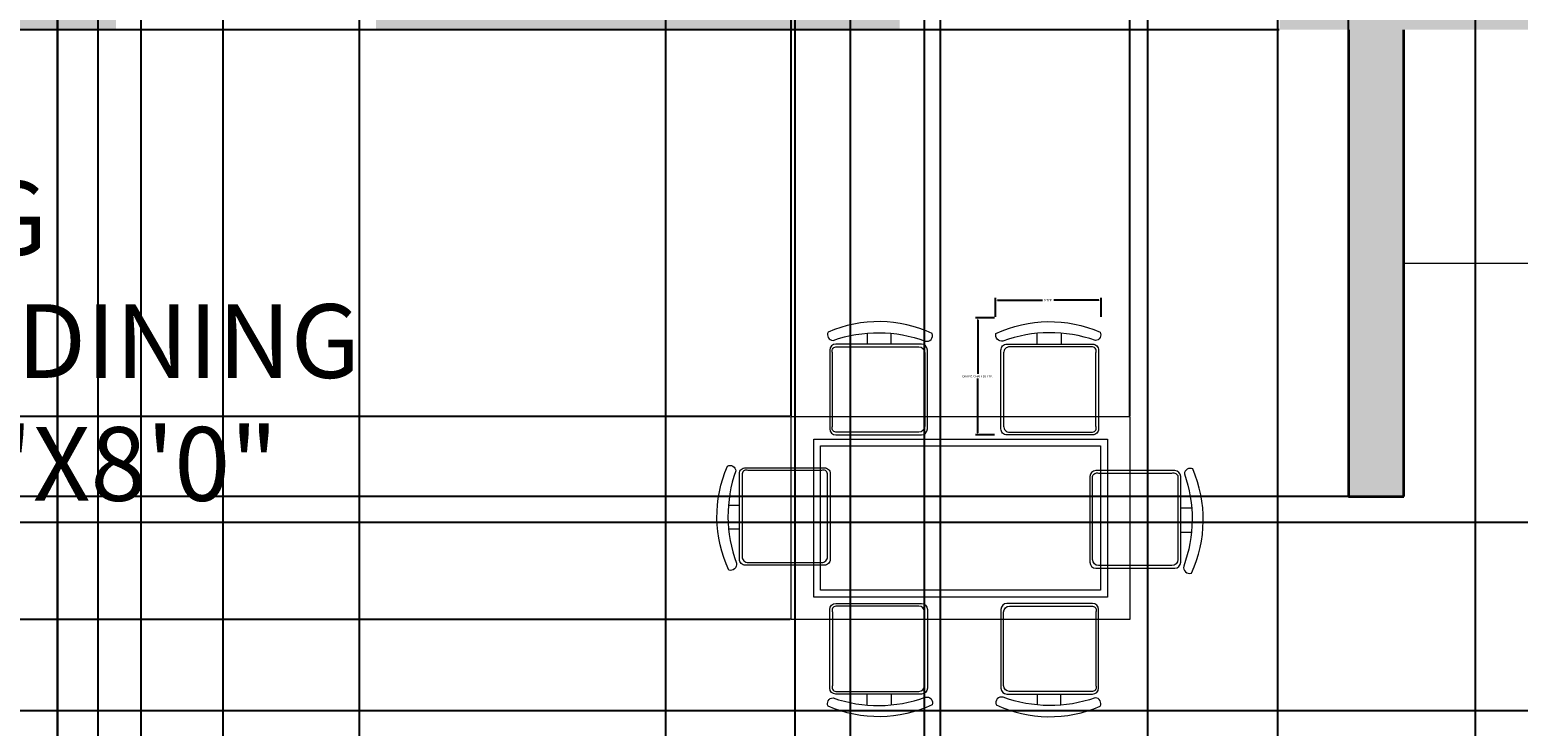
# Model space of a CAD drawing. Units: inches. Extents: x 2606 to 3027, y 1906 to 2463.
# Tile 6 of 10: x 2785 to 2906, y 2196 to 2253. Entities that reach past the tile are written whole.
import ezdxf

# ---------------------------------------------------------------- set-up
doc = ezdxf.new("R2010")
doc.units = ezdxf.units.IN
for name, color, linetype, lineweight in [('A-ANNO-DIMS', 2, 'Continuous', 18), ('A-AREA-IDEN', 7, 'Continuous', 18), ('A-FLOR-CASE', 8, 'Continuous', 18), ('A-FURN', 8, 'Continuous', 13), ('A-WALL', 7, 'Continuous', 35)]:
    doc.layers.add(name, color=color, linetype=linetype, lineweight=lineweight)
doc.layers.add('A-WALL-PATT', color=251, linetype='Continuous', lineweight=13, true_color=0x636466)
doc.styles.get("Standard").update_dxf_attribs({"font": 'arial.ttf'})
doc.dimstyles.get("Standard").update_dxf_attribs({"dimtxt": 0.18, "dimasz": 0.18, "dimexe": 0.18, "dimexo": 0.0625, "dimgap": 0.09, "dimtad": 0, "dimtih": 1, "dimtoh": 1, "dimdec": 4, "dimzin": 0, "dimdsep": 46, "dimtxsty": 'Standard', "dimcen": 0.09, "dimadec": 0, "dimazin": 0, "dimtfac": 1, "dimtdec": 4, "dimtofl": 0, "dimtmove": 0, "dimatfit": 3, "dimfxl": 1, "dimtolj": 1, "dimtzin": 0, "dimarcsym": 0})

# ---------------------------------------------------------------- blocks, each defined once
blk = doc.blocks.new('CHAIR-DINING')
for points in [[(0.59, 7.63, -0.578392), (0.02, 8.25, -0.214524), (8.49, 8.36, -0.552014), (8.1, 7.68, 0.175809), (0.59, 7.63)], [(7.88, 7.38, -0.414214), (8.36, 6.89), (8.36, 0.49, -0.414214), (7.88, 0), (0.91, 0, -0.414214), (0.42, 0.49), (0.42, 6.89, -0.414214), (0.91, 7.38), (7.88, 7.38)], [(3.36, 7.38), (3.36, 8.26, 0.064759)]]:
    blk.add_lwpolyline(points, format="xyb")
blk.add_lwpolyline([(5.31, 8.28), (5.31, 7.38)])
blk.add_lwpolyline([(7.87, 7.16), (1.13, 7.16, 0.414214), (0.64, 6.67), (0.64, 0.71, 0.414214), (1.13, 0.22), (7.87, 0.22, 0.512069), (8.14, 0.71), (8.14, 6.67, 0.512069)], format="xyb", close=True)
blk = doc.blocks.new('*D23')
at = {"layer": 'A-ANNO-DIMS', "color": 0, "lineweight": -2, "transparency": 16777216}
for p, q in [((2863.77, 2229.68), (2862.22, 2229.68)), ((2862.4, 2229.5), (2862.4, 2225.1)), ((2862.4, 2220.32), (2862.4, 2224.73)), ((2863.77, 2220.14), (2862.22, 2220.14))]:
    blk.add_line(p, q, dxfattribs=at)
at = {"layer": 'A-ANNO-DIMS', "color": 0, "transparency": 16777216}
for points in [[(2862.37, 2229.5), (2862.43, 2229.5), (2862.4, 2229.68)], [(2862.37, 2220.32), (2862.43, 2220.32), (2862.4, 2220.14)]]:
    blk.add_solid(points, dxfattribs=at)
at = {"layer": 'Defpoints', "color": 0, "transparency": 16777216}
for p in [(2862.4, 2229.68), (2863.84, 2229.68), (2863.84, 2220.14)]:
    blk.add_point(p, dxfattribs=at)
at = {"layer": 'A-ANNO-DIMS', "color": 0, "transparency": 16777216, "insert": (2862.4, 2224.91), "char_height": 0.18, "attachment_point": 5}
blk.add_mtext('\\A1;DINING CHAIR 10 TYP.', dxfattribs=at)
blk = doc.blocks.new('*D24')
at = {"layer": 'A-ANNO-DIMS', "color": 0, "lineweight": -2, "transparency": 16777216}
for p, q in [((2863.84, 2229.75), (2863.84, 2231.29)), ((2864.02, 2231.11), (2867.68, 2231.11)), ((2872.25, 2231.11), (2868.59, 2231.11)), ((2872.43, 2229.75), (2872.43, 2231.29))]:
    blk.add_line(p, q, dxfattribs=at)
at = {"layer": 'A-ANNO-DIMS', "color": 0, "transparency": 16777216}
for points in [[(2864.02, 2231.14), (2864.02, 2231.08), (2863.84, 2231.11)], [(2872.25, 2231.14), (2872.25, 2231.08), (2872.43, 2231.11)]]:
    blk.add_solid(points, dxfattribs=at)
at = {"layer": 'Defpoints', "color": 0, "transparency": 16777216}
for p in [(2872.43, 2231.11), (2863.84, 2229.68), (2872.43, 2229.68)]:
    blk.add_point(p, dxfattribs=at)
at = {"layer": 'A-ANNO-DIMS', "color": 0, "transparency": 16777216, "insert": (2868.13, 2231.11), "char_height": 0.18, "attachment_point": 5}
blk.add_mtext('\\A1;9 TYP.', dxfattribs=at)
blk = doc.blocks.new('*D34')
at = {"layer": 'A-ANNO-DIMS', "color": 0, "lineweight": -2, "transparency": 16777216}
for p, q in [((2787.56, 2118.27), (2787.56, 2433.99)), ((2787.74, 2433.81), (2817.34, 2433.81)), ((2847.38, 2433.81), (2817.78, 2433.81)), ((2847.56, 2118.27), (2847.56, 2433.99))]:
    blk.add_line(p, q, dxfattribs=at)
at = {"layer": 'A-ANNO-DIMS', "color": 0, "transparency": 16777216}
for points in [[(2787.74, 2433.84), (2787.74, 2433.78), (2787.56, 2433.81)], [(2847.38, 2433.84), (2847.38, 2433.78), (2847.56, 2433.81)]]:
    blk.add_solid(points, dxfattribs=at)
at = {"layer": 'Defpoints', "color": 0, "transparency": 16777216}
for p in [(2847.56, 2433.81), (2787.56, 2118.21), (2847.56, 2118.21)]:
    blk.add_point(p, dxfattribs=at)
at = {"layer": 'A-ANNO-DIMS', "color": 0, "transparency": 16777216, "insert": (2817.56, 2433.81), "char_height": 0.18, "attachment_point": 5}
blk.add_mtext('\\A1;60', dxfattribs=at)
blk = doc.blocks.new('*D35')
at = {"layer": 'A-ANNO-DIMS', "color": 0, "lineweight": -2, "transparency": 16777216}
for p, q in [((2801.04, 1993.17), (2801.04, 2433.99)), ((2801.22, 2433.81), (2818.82, 2433.81)), ((2836.86, 2433.81), (2819.26, 2433.81)), ((2837.04, 1993.17), (2837.04, 2433.99))]:
    blk.add_line(p, q, dxfattribs=at)
at = {"layer": 'A-ANNO-DIMS', "color": 0, "transparency": 16777216}
for points in [[(2801.22, 2433.84), (2801.22, 2433.78), (2801.04, 2433.81)], [(2836.86, 2433.84), (2836.86, 2433.78), (2837.04, 2433.81)]]:
    blk.add_solid(points, dxfattribs=at)
at = {"layer": 'Defpoints', "color": 0, "transparency": 16777216}
for p in [(2837.04, 2433.81), (2801.04, 1993.11), (2837.04, 1993.11)]:
    blk.add_point(p, dxfattribs=at)
at = {"layer": 'A-ANNO-DIMS', "color": 0, "transparency": 16777216, "insert": (2819.04, 2433.81), "char_height": 0.18, "attachment_point": 5}
blk.add_mtext('\\A1;36', dxfattribs=at)
blk = doc.blocks.new('*D36')
at = {"layer": 'A-ANNO-DIMS', "color": 0, "lineweight": -2, "transparency": 16777216}
for p, q in [((2787.56, 1993.17), (2787.56, 2433.99)), ((2787.74, 2433.81), (2793.85, 2433.81)), ((2800.86, 2433.81), (2794.76, 2433.81)), ((2801.04, 1993.17), (2801.04, 2433.99))]:
    blk.add_line(p, q, dxfattribs=at)
at = {"layer": 'A-ANNO-DIMS', "color": 0, "transparency": 16777216}
for points in [[(2787.74, 2433.84), (2787.74, 2433.78), (2787.56, 2433.81)], [(2800.86, 2433.84), (2800.86, 2433.78), (2801.04, 2433.81)]]:
    blk.add_solid(points, dxfattribs=at)
at = {"layer": 'Defpoints', "color": 0, "transparency": 16777216}
for p in [(2787.56, 2433.81), (2787.56, 1993.11), (2801.04, 1993.11)]:
    blk.add_point(p, dxfattribs=at)
at = {"layer": 'A-ANNO-DIMS', "color": 0, "transparency": 16777216, "insert": (2794.3, 2433.81), "char_height": 0.18, "attachment_point": 5}
blk.add_mtext('\\A1;13.478', dxfattribs=at)
blk = doc.blocks.new('*D38')
at = {"layer": 'A-ANNO-DIMS', "color": 0, "lineweight": -2, "transparency": 16777216}
for p, q in [((2783.06, 1993.17), (2783.06, 2433.99)), ((2783.24, 2433.81), (2785.05, 2433.81)), ((2787.38, 2433.81), (2785.57, 2433.81)), ((2787.56, 1993.17), (2787.56, 2433.99))]:
    blk.add_line(p, q, dxfattribs=at)
at = {"layer": 'A-ANNO-DIMS', "color": 0, "transparency": 16777216}
for points in [[(2783.24, 2433.84), (2783.24, 2433.78), (2783.06, 2433.81)], [(2787.38, 2433.84), (2787.38, 2433.78), (2787.56, 2433.81)]]:
    blk.add_solid(points, dxfattribs=at)
at = {"layer": 'Defpoints', "color": 0, "transparency": 16777216}
for p in [(2787.56, 2433.81), (2783.06, 1993.11), (2787.56, 1993.11)]:
    blk.add_point(p, dxfattribs=at)
at = {"layer": 'A-ANNO-DIMS', "color": 0, "transparency": 16777216, "insert": (2785.31, 2433.81), "char_height": 0.18, "attachment_point": 5}
blk.add_mtext('\\A1;4.5', dxfattribs=at)
blk = doc.blocks.new('*D43')
at = {"layer": 'A-ANNO-DIMS', "color": 0, "lineweight": -2, "transparency": 16777216}
for p, q in [((2794.34, 2257.55), (2794.34, 1965.23)), ((2812.09, 2257.55), (2812.09, 1965.23)), ((2794.52, 1965.41), (2802.76, 1965.41)), ((2811.91, 1965.41), (2803.67, 1965.41))]:
    blk.add_line(p, q, dxfattribs=at)
at = {"layer": 'A-ANNO-DIMS', "color": 0, "transparency": 16777216}
for points in [[(2794.52, 1965.44), (2794.52, 1965.38), (2794.34, 1965.41)], [(2811.91, 1965.44), (2811.91, 1965.38), (2812.09, 1965.41)]]:
    blk.add_solid(points, dxfattribs=at)
at = {"layer": 'Defpoints', "color": 0, "transparency": 16777216}
for p in [(2794.34, 2257.61), (2812.09, 2257.61), (2812.09, 1965.41)]:
    blk.add_point(p, dxfattribs=at)
at = {"layer": 'A-ANNO-DIMS', "color": 0, "transparency": 16777216, "insert": (2803.22, 1965.41), "char_height": 0.18, "attachment_point": 5}
blk.add_mtext('\\A1;17.756', dxfattribs=at)
blk = doc.blocks.new('*D46')
at = {"layer": 'A-ANNO-DIMS', "color": 0, "lineweight": -2, "transparency": 16777216}
for p, q in [((2859.37, 2154.92), (2859.37, 2433.99)), ((2859.55, 2433.81), (2872.63, 2433.81)), ((2886.63, 2433.81), (2873.56, 2433.81)), ((2886.81, 2157.17), (2886.81, 2433.99))]:
    blk.add_line(p, q, dxfattribs=at)
at = {"layer": 'A-ANNO-DIMS', "color": 0, "transparency": 16777216}
for points in [[(2859.55, 2433.84), (2859.55, 2433.78), (2859.37, 2433.81)], [(2886.63, 2433.84), (2886.63, 2433.78), (2886.81, 2433.81)]]:
    blk.add_solid(points, dxfattribs=at)
at = {"layer": 'Defpoints', "color": 0, "transparency": 16777216}
for p in [(2886.81, 2433.81), (2886.81, 2157.11), (2859.37, 2154.86)]:
    blk.add_point(p, dxfattribs=at)
at = {"layer": 'A-ANNO-DIMS', "color": 0, "transparency": 16777216, "insert": (2873.09, 2433.81), "char_height": 0.18, "attachment_point": 5}
blk.add_mtext('\\A1;27.443', dxfattribs=at)
blk = doc.blocks.new('*D48')
at = {"layer": 'A-ANNO-DIMS', "color": 0, "lineweight": -2, "transparency": 16777216}
for p, q in [((2858.07, 2028.17), (2858.07, 2433.99)), ((2858.25, 2433.81), (2866.77, 2433.81)), ((2876.06, 2433.81), (2867.54, 2433.81)), ((2876.24, 2028.17), (2876.24, 2433.99))]:
    blk.add_line(p, q, dxfattribs=at)
at = {"layer": 'A-ANNO-DIMS', "color": 0, "transparency": 16777216}
for points in [[(2858.25, 2433.84), (2858.25, 2433.78), (2858.07, 2433.81)], [(2876.06, 2433.84), (2876.06, 2433.78), (2876.24, 2433.81)]]:
    blk.add_solid(points, dxfattribs=at)
at = {"layer": 'Defpoints', "color": 0, "transparency": 16777216}
for p in [(2876.24, 2433.81), (2858.07, 2028.11), (2876.24, 2028.11)]:
    blk.add_point(p, dxfattribs=at)
at = {"layer": 'A-ANNO-DIMS', "color": 0, "transparency": 16777216, "insert": (2867.16, 2433.81), "char_height": 0.18, "attachment_point": 5}
blk.add_mtext('\\A1;18.17', dxfattribs=at)
blk = doc.blocks.new('*D52')
at = {"layer": 'A-ANNO-DIMS', "color": 0, "lineweight": -2, "transparency": 16777216}
for p, q in [((2787.56, 2257.55), (2787.56, 1965.23)), ((2794.34, 2257.55), (2794.34, 1965.23)), ((2787.74, 1965.41), (2790.56, 1965.41)), ((2794.16, 1965.41), (2791.34, 1965.41))]:
    blk.add_line(p, q, dxfattribs=at)
at = {"layer": 'A-ANNO-DIMS', "color": 0, "transparency": 16777216}
for points in [[(2787.74, 1965.44), (2787.74, 1965.38), (2787.56, 1965.41)], [(2794.16, 1965.44), (2794.16, 1965.38), (2794.34, 1965.41)]]:
    blk.add_solid(points, dxfattribs=at)
at = {"layer": 'Defpoints', "color": 0, "transparency": 16777216}
for p in [(2787.56, 2257.61), (2794.34, 2257.61), (2794.34, 1965.41)]:
    blk.add_point(p, dxfattribs=at)
at = {"layer": 'A-ANNO-DIMS', "color": 0, "transparency": 16777216, "insert": (2790.95, 1965.41), "char_height": 0.18, "attachment_point": 5}
blk.add_mtext('\\A1;6.776', dxfattribs=at)
blk = doc.blocks.new('*D55')
at = {"layer": 'A-ANNO-DIMS', "color": 0, "lineweight": -2, "transparency": 16777216}
for p, q in [((2852.06, 2152.67), (2852.06, 2433.99)), ((2852.24, 2433.81), (2855.32, 2433.81)), ((2859.19, 2433.81), (2856.11, 2433.81)), ((2859.37, 2154.92), (2859.37, 2433.99))]:
    blk.add_line(p, q, dxfattribs=at)
at = {"layer": 'A-ANNO-DIMS', "color": 0, "transparency": 16777216}
for points in [[(2852.24, 2433.84), (2852.24, 2433.78), (2852.06, 2433.81)], [(2859.19, 2433.84), (2859.19, 2433.78), (2859.37, 2433.81)]]:
    blk.add_solid(points, dxfattribs=at)
at = {"layer": 'Defpoints', "color": 0, "transparency": 16777216}
for p in [(2859.37, 2433.81), (2859.37, 2154.86), (2852.06, 2152.61)]:
    blk.add_point(p, dxfattribs=at)
at = {"layer": 'A-ANNO-DIMS', "color": 0, "transparency": 16777216, "insert": (2855.72, 2433.81), "char_height": 0.18, "attachment_point": 5}
blk.add_mtext('\\A1;7.306', dxfattribs=at)
blk = doc.blocks.new('*D57')
at = {"layer": 'A-ANNO-DIMS', "color": 0, "lineweight": -2, "transparency": 16777216}
for p, q in [((2876.24, 2028.17), (2876.24, 2433.99)), ((2876.42, 2433.81), (2889.17, 2433.81)), ((2902.71, 2433.81), (2889.96, 2433.81)), ((2902.89, 2028.17), (2902.89, 2433.99))]:
    blk.add_line(p, q, dxfattribs=at)
at = {"layer": 'A-ANNO-DIMS', "color": 0, "transparency": 16777216}
for points in [[(2876.42, 2433.84), (2876.42, 2433.78), (2876.24, 2433.81)], [(2902.71, 2433.84), (2902.71, 2433.78), (2902.89, 2433.81)]]:
    blk.add_solid(points, dxfattribs=at)
at = {"layer": 'Defpoints', "color": 0, "transparency": 16777216}
for p in [(2902.89, 2433.81), (2876.24, 2028.11), (2902.89, 2028.11)]:
    blk.add_point(p, dxfattribs=at)
at = {"layer": 'A-ANNO-DIMS', "color": 0, "transparency": 16777216, "insert": (2889.57, 2433.81), "char_height": 0.18, "attachment_point": 5}
blk.add_mtext('\\A1;26.65', dxfattribs=at)
blk = doc.blocks.new('*D59')
at = {"layer": 'A-ANNO-DIMS', "color": 0, "lineweight": -2, "transparency": 16777216}
for p, q in [((2726.47, 2213.03), (3000.44, 2213.03)), ((3000.26, 2212.85), (3000.26, 2205.56)), ((3000.26, 2197.9), (3000.26, 2205.2)), ((2726.47, 2197.72), (3000.44, 2197.72))]:
    blk.add_line(p, q, dxfattribs=at)
at = {"layer": 'A-ANNO-DIMS', "color": 0, "transparency": 16777216}
for points in [[(3000.23, 2212.85), (3000.29, 2212.85), (3000.26, 2213.03)], [(3000.23, 2197.9), (3000.29, 2197.9), (3000.26, 2197.72)]]:
    blk.add_solid(points, dxfattribs=at)
at = {"layer": 'Defpoints', "color": 0, "transparency": 16777216}
for p in [(2726.4, 2213.03), (3000.26, 2213.03), (2726.4, 2197.72)]:
    blk.add_point(p, dxfattribs=at)
at = {"layer": 'A-ANNO-DIMS', "color": 0, "transparency": 16777216, "insert": (3000.26, 2205.38), "char_height": 0.18, "attachment_point": 5}
blk.add_mtext('\\A1;15.31', dxfattribs=at)
blk = doc.blocks.new('*D61')
at = {"layer": 'A-ANNO-DIMS', "color": 0, "lineweight": -2, "transparency": 16777216}
for p, q in [((2696.29, 2197.72), (3000.44, 2197.72)), ((3000.26, 2197.54), (3000.26, 2190.63)), ((3000.26, 2183.36), (3000.26, 2190.27)), ((2696.84, 2183.18), (3000.44, 2183.18))]:
    blk.add_line(p, q, dxfattribs=at)
at = {"layer": 'A-ANNO-DIMS', "color": 0, "transparency": 16777216}
for points in [[(3000.23, 2197.54), (3000.29, 2197.54), (3000.26, 2197.72)], [(3000.23, 2183.36), (3000.29, 2183.36), (3000.26, 2183.18)]]:
    blk.add_solid(points, dxfattribs=at)
at = {"layer": 'Defpoints', "color": 0, "transparency": 16777216}
for p in [(2696.23, 2197.72), (3000.26, 2197.72), (2696.78, 2183.18)]:
    blk.add_point(p, dxfattribs=at)
at = {"layer": 'A-ANNO-DIMS', "color": 0, "transparency": 16777216, "insert": (3000.26, 2190.45), "char_height": 0.18, "attachment_point": 5}
blk.add_mtext('\\A1;14.545', dxfattribs=at)
blk = doc.blocks.new('*D68')
at = {"layer": 'A-ANNO-DIMS', "color": 0, "lineweight": -2, "transparency": 16777216}
for p, q in [((2897, 2215.13), (2634.68, 2215.13)), ((2634.86, 2214.95), (2634.86, 2194.85)), ((2634.86, 2174.38), (2634.86, 2194.48)), ((2897, 2174.2), (2634.68, 2174.2))]:
    blk.add_line(p, q, dxfattribs=at)
at = {"layer": 'A-ANNO-DIMS', "color": 0, "transparency": 16777216}
for points in [[(2634.83, 2214.95), (2634.89, 2214.95), (2634.86, 2215.13)], [(2634.83, 2174.38), (2634.89, 2174.38), (2634.86, 2174.2)]]:
    blk.add_solid(points, dxfattribs=at)
at = {"layer": 'Defpoints', "color": 0, "transparency": 16777216}
for p in [(2897.06, 2215.13), (2634.86, 2174.2), (2897.06, 2174.2)]:
    blk.add_point(p, dxfattribs=at)
at = {"layer": 'A-ANNO-DIMS', "color": 0, "transparency": 16777216, "insert": (2634.86, 2194.66), "char_height": 0.18, "attachment_point": 5}
blk.add_mtext('\\A1;40.94', dxfattribs=at)
blk = doc.blocks.new('*D70')
at = {"layer": 'A-ANNO-DIMS', "color": 0, "lineweight": -2, "transparency": 16777216}
for p, q in [((2847.23, 2221.7), (2847.23, 2433.99)), ((2847.41, 2433.81), (2860.54, 2433.81)), ((2874.6, 2433.81), (2861.47, 2433.81)), ((2874.78, 2221.7), (2874.78, 2433.99))]:
    blk.add_line(p, q, dxfattribs=at)
at = {"layer": 'A-ANNO-DIMS', "color": 0, "transparency": 16777216}
for points in [[(2847.41, 2433.84), (2847.41, 2433.78), (2847.23, 2433.81)], [(2874.6, 2433.84), (2874.6, 2433.78), (2874.78, 2433.81)]]:
    blk.add_solid(points, dxfattribs=at)
at = {"layer": 'Defpoints', "color": 0, "transparency": 16777216}
for p in [(2874.78, 2433.81), (2847.23, 2221.64), (2874.78, 2221.64)]:
    blk.add_point(p, dxfattribs=at)
at = {"layer": 'A-ANNO-DIMS', "color": 0, "transparency": 16777216, "insert": (2861, 2433.81), "char_height": 0.18, "attachment_point": 5}
blk.add_mtext('\\A1;27.555', dxfattribs=at)
blk = doc.blocks.new('*D71')
at = {"layer": 'A-ANNO-DIMS', "color": 0, "lineweight": -2, "transparency": 16777216}
for p, q in [((2847.16, 2221.64), (2634.68, 2221.64)), ((2634.86, 2221.46), (2634.86, 2213.56)), ((2634.86, 2205.29), (2634.86, 2213.19)), ((2847.16, 2205.11), (2634.68, 2205.11))]:
    blk.add_line(p, q, dxfattribs=at)
at = {"layer": 'A-ANNO-DIMS', "color": 0, "transparency": 16777216}
for points in [[(2634.83, 2221.46), (2634.89, 2221.46), (2634.86, 2221.64)], [(2634.83, 2205.29), (2634.89, 2205.29), (2634.86, 2205.11)]]:
    blk.add_solid(points, dxfattribs=at)
at = {"layer": 'Defpoints', "color": 0, "transparency": 16777216}
for p in [(2847.23, 2221.64), (2634.86, 2205.11), (2847.23, 2205.11)]:
    blk.add_point(p, dxfattribs=at)
at = {"layer": 'A-ANNO-DIMS', "color": 0, "transparency": 16777216, "insert": (2634.86, 2213.37), "char_height": 0.18, "attachment_point": 5}
blk.add_mtext('\\A1;16.533', dxfattribs=at)
blk = doc.blocks.new('*D72')
at = {"layer": 'A-ANNO-DIMS', "color": 0, "lineweight": -2, "transparency": 16777216}
for p, q in [((2874.78, 2221.7), (2874.78, 2433.99)), ((2874.96, 2433.81), (2883.22, 2433.81)), ((2892.38, 2433.81), (2884.13, 2433.81)), ((2892.56, 2215.2), (2892.56, 2433.99))]:
    blk.add_line(p, q, dxfattribs=at)
at = {"layer": 'A-ANNO-DIMS', "color": 0, "transparency": 16777216}
for points in [[(2874.96, 2433.84), (2874.96, 2433.78), (2874.78, 2433.81)], [(2892.38, 2433.84), (2892.38, 2433.78), (2892.56, 2433.81)]]:
    blk.add_solid(points, dxfattribs=at)
at = {"layer": 'Defpoints', "color": 0, "transparency": 16777216}
for p in [(2892.56, 2433.81), (2874.78, 2221.64), (2892.56, 2215.13)]:
    blk.add_point(p, dxfattribs=at)
at = {"layer": 'A-ANNO-DIMS', "color": 0, "transparency": 16777216, "insert": (2883.67, 2433.81), "char_height": 0.18, "attachment_point": 5}
blk.add_mtext('\\A1;17.783', dxfattribs=at)
blk = doc.blocks.new('*D73')
at = {"layer": 'A-ANNO-DIMS', "color": 0, "lineweight": -2, "transparency": 16777216}
for p, q in [((2886.91, 2253.11), (2634.68, 2253.11)), ((2634.86, 2252.93), (2634.86, 2237.56)), ((2634.86, 2221.82), (2634.86, 2237.19)), ((2847.16, 2221.64), (2634.68, 2221.64))]:
    blk.add_line(p, q, dxfattribs=at)
at = {"layer": 'A-ANNO-DIMS', "color": 0, "transparency": 16777216}
for points in [[(2634.83, 2252.93), (2634.89, 2252.93), (2634.86, 2253.11)], [(2634.83, 2221.82), (2634.89, 2221.82), (2634.86, 2221.64)]]:
    blk.add_solid(points, dxfattribs=at)
at = {"layer": 'Defpoints', "color": 0, "transparency": 16777216}
for p in [(2634.86, 2253.11), (2886.97, 2253.11), (2847.23, 2221.64)]:
    blk.add_point(p, dxfattribs=at)
at = {"layer": 'A-ANNO-DIMS', "color": 0, "transparency": 16777216, "insert": (2634.86, 2237.37), "char_height": 0.18, "attachment_point": 5}
blk.add_mtext('\\A1;31.47', dxfattribs=at)
blk = doc.blocks.new('*D83')
at = {"layer": 'A-ANNO-DIMS', "color": 0, "lineweight": -2, "transparency": 16777216}
for p, q in [((2787.56, 2327.05), (2787.56, 1965.23)), ((2790.85, 2327.05), (2790.85, 1965.23)), ((2787.74, 1965.41), (2788.88, 1965.41)), ((2790.67, 1965.41), (2789.53, 1965.41))]:
    blk.add_line(p, q, dxfattribs=at)
at = {"layer": 'A-ANNO-DIMS', "color": 0, "transparency": 16777216}
for points in [[(2787.74, 1965.44), (2787.74, 1965.38), (2787.56, 1965.41)], [(2790.67, 1965.44), (2790.67, 1965.38), (2790.85, 1965.41)]]:
    blk.add_solid(points, dxfattribs=at)
at = {"layer": 'Defpoints', "color": 0, "transparency": 16777216}
for p in [(2787.56, 2327.11), (2790.85, 2327.11), (2790.85, 1965.41)]:
    blk.add_point(p, dxfattribs=at)
at = {"layer": 'A-ANNO-DIMS', "color": 0, "transparency": 16777216, "insert": (2789.21, 1965.41), "char_height": 0.18, "attachment_point": 5}
blk.add_mtext('\\A1;3.29', dxfattribs=at)

msp = doc.modelspace()

# ---------------------------------------------------------------- hatches: boundary and pattern name
at = {"layer": 'A-WALL-PATT'}
h = msp.add_hatch(color=256, dxfattribs=at)
h.dxf.hatch_style = 1
h.paths.add_polyline_path([(2667.063, 2401.6097), (2691.9697, 2401.6097), (2691.9697, 2406.1097), (2691.9697, 2410.6097), (2658.063, 2410.6097), (2658.063, 2238.7051), (2667.063, 2238.7051)])
h.paths.add_polyline_path([(2804.9965, 2406.1097), (2804.9965, 2410.6097), (2751.9697, 2410.6097), (2751.9697, 2401.6097), (2783.063, 2401.6097), (2783.063, 2257.6097), (2778.6739, 2257.6097), (2778.6739, 2253.1097), (2792.3386, 2253.1097), (2792.3386, 2255.3597), (2792.3386, 2257.6097), (2787.563, 2257.6097), (2787.563, 2327.1097), (2847.563, 2327.1097), (2847.563, 2331.6097), (2787.563, 2331.6097), (2787.563, 2401.6097), (2804.9965, 2401.6097)])
h.paths.add_polyline_path([(2889.6183, 2406.1097), (2889.6183, 2410.6097), (2828.9965, 2410.6097), (2828.9965, 2401.6097), (2831.8174, 2401.6097), (2847.563, 2401.6097), (2847.563, 2357.8311), (2849.813, 2357.8311), (2852.063, 2357.8311), (2852.063, 2401.6097), (2889.6183, 2401.6097)])
h.paths.add_polyline_path([(2977.063, 2410.6097), (2949.6183, 2410.6097), (2949.6183, 2401.6097), (2968.063, 2401.6097), (2968.063, 2157.1097), (2897.063, 2157.1097), (2897.063, 2174.1966), (2892.563, 2174.1966), (2892.563, 2157.1097), (2886.8122, 2157.1097), (2886.8122, 2152.6097), (2968.063, 2152.6097), (2968.063, 2032.6097), (2950.8911, 2032.6097), (2950.8911, 2028.1097), (2968.063, 2028.1097), (2968.063, 1993.1097), (2852.063, 1993.1097), (2852.063, 2028.1097), (2856.0743, 2028.1097), (2856.0743, 2030.3597), (2856.0743, 2032.6097), (2852.063, 2032.6097), (2852.063, 2152.6097), (2857.369, 2152.6097), (2857.369, 2154.8597), (2857.369, 2157.1097), (2847.563, 2157.1097), (2847.563, 2152.6097), (2847.563, 1993.1097), (2837.0415, 1993.1097), (2837.0415, 1988.6097), (2977.063, 1988.6097)])
h.paths.add_polyline_path([(2968.063, 2257.6097), (2886.9679, 2257.6097), (2886.9679, 2253.1097), (2892.563, 2253.1097), (2892.563, 2215.1332), (2897.063, 2215.1332), (2897.063, 2253.1097), (2968.063, 2253.1097)], flags=17)
h.paths.add_polyline_path([(2856.057, 2255.3597), (2856.057, 2257.6097), (2852.063, 2257.6097), (2852.063, 2336.7476), (2849.813, 2336.7476), (2847.563, 2336.7476), (2847.563, 2331.6097), (2847.563, 2327.1097), (2847.563, 2257.6097), (2813.482, 2257.6097), (2813.482, 2253.1097), (2856.057, 2253.1097)])
h.paths.add_polyline_path([(2748.8874, 2255.3597), (2748.8874, 2257.6097), (2667.063, 2257.6097), (2667.063, 2253.1097), (2748.8874, 2253.1097)])
h.paths.add_polyline_path([(2667.063, 2152.6097), (2744.8238, 2152.6097), (2744.8238, 2154.8597), (2744.8238, 2157.1097), (2667.063, 2157.1097), (2667.063, 2178.7051), (2658.063, 2178.7051), (2658.063, 1988.6097), (2801.0415, 1988.6097), (2801.0415, 1990.8597), (2801.0415, 1993.1097), (2787.563, 1993.1097), (2787.563, 2157.1097), (2777.1295, 2157.1097), (2777.1295, 2152.6097), (2783.063, 2152.6097), (2783.063, 2032.6097), (2778.4484, 2032.6097), (2778.4484, 2028.1097), (2783.063, 2028.1097), (2783.063, 1993.1097), (2667.063, 1993.1097), (2667.063, 2028.1097), (2680.1652, 2028.1097), (2680.1652, 2030.3597), (2680.1652, 2032.6097), (2667.063, 2032.6097)])
h.paths.add_polyline_path([(2755.4074, 2032.6097), (2728.1652, 2032.6097), (2728.1652, 2028.1097), (2755.4074, 2028.1097), (2755.4074, 2030.3597)], flags=17)
h.paths.add_polyline_path([(2902.8911, 2030.3597), (2902.8911, 2032.6097), (2877.6885, 2032.6097), (2877.6885, 2028.1097), (2902.8911, 2028.1097)], flags=17)
h.paths.add_polyline_path([(2810.2211, 2267.221), (2851.2716, 2267.221), (2851.2716, 2289.6098), (2810.2211, 2289.6098)], flags=9)

# ---------------------------------------------------------------- linework, layer by layer
at = {"layer": 'A-FLOR-CASE'}
msp.add_line((2897.063, 2234.1214), (2944.3333, 2234.1214), dxfattribs=at)
at = {"layer": 'A-FURN'}
for points in [[(2850.6334, 2227.8254, -0.17580919), (2858.1386, 2227.7686, 0.57839206), (2858.7071, 2228.3938, 0.21452438), (2850.2354, 2228.5075, 0.55201397), (2850.6334, 2227.8254, -0.06507904)], [(2855.3728, 2227.5242), (2855.3728, 2228.4054, -0.06475861)], [(2857.8202, 2227.5242), (2850.8526, 2227.5242, 0.41421356), (2850.3651, 2227.0368), (2850.3651, 2220.6302, 0.41421356), (2850.8526, 2220.1427), (2857.8202, 2220.1427, 0.41421356), (2858.3076, 2220.6302), (2858.3076, 2227.0368, 0.41421356), (2857.8202, 2227.5242)], [(2878.9056, 2216.7489, 0.41421356), (2878.4182, 2217.2363), (2872.0116, 2217.2363, 0.41421356), (2871.5242, 2216.7489), (2871.5242, 2209.7813, 0.41421356), (2872.0116, 2209.2938), (2878.4182, 2209.2938, 0.41421356), (2878.9056, 2209.7813), (2878.9056, 2216.7489)], [(2879.2069, 2216.9681, -0.17580919), (2879.15, 2209.4629, 0.57839206), (2879.7752, 2208.8943, 0.21452438), (2879.8889, 2217.3661, 0.55201397), (2879.2069, 2216.9681, -0.06507904)], [(2878.9056, 2212.2286), (2879.7868, 2212.2286, -0.06475861)], [(2857.8202, 2199.0455), (2850.8526, 2199.0455, -0.41421356), (2850.3651, 2199.533), (2850.3651, 2205.9395, -0.41421356), (2850.8526, 2206.427), (2857.8202, 2206.427, -0.41421356), (2858.3076, 2205.9395), (2858.3076, 2199.533, -0.41421356), (2857.8202, 2199.0455)], [(2871.743, 2199.0455, 0.41421356), (2872.2304, 2199.533), (2872.2304, 2205.9395, 0.41421356), (2871.743, 2206.427), (2864.7754, 2206.427, 0.41421356), (2864.2879, 2205.9395), (2864.2879, 2199.533, 0.41421356), (2864.7754, 2199.0455), (2871.743, 2199.0455)], [(2858.1386, 2198.8011, -0.57839206), (2858.7071, 2198.1759, -0.21452438), (2850.2354, 2198.0622, -0.55201397), (2850.6334, 2198.7443, 0.17580929), (2858.1386, 2198.8011)], [(2855.3728, 2199.0455), (2855.3728, 2198.1643, 0.06475861)], [(2871.9622, 2198.7443, -0.17580928), (2864.457, 2198.8011, 0.57839206), (2863.8884, 2198.1759, 0.21452438), (2872.3602, 2198.0622, 0.55201397), (2871.9622, 2198.7443, -0.06507904)], [(2867.2228, 2199.0455), (2867.2228, 2198.1643, -0.06475861)]]:
    msp.add_lwpolyline(points, format="xyb", dxfattribs=at)
for points in [[(2853.4225, 2228.4214), (2853.4225, 2227.5242)], [(2879.8028, 2214.179), (2878.9056, 2214.179)], [(2853.4225, 2198.1483), (2853.4225, 2199.0455)], [(2869.1731, 2198.1483), (2869.1731, 2199.0455)]]:
    msp.add_lwpolyline(points, dxfattribs=at)
for points in [[(2850.8555, 2227.3046), (2857.6005, 2227.3046, -0.41421356), (2858.088, 2226.8171), (2858.088, 2220.8498, -0.41421356), (2857.6005, 2220.3623), (2850.8555, 2220.3623, -0.51206948), (2850.5847, 2220.8498), (2850.5847, 2226.8171, -0.51206948)], [(2878.686, 2216.7459), (2878.686, 2210.0009, -0.41421356), (2878.1986, 2209.5134), (2872.2312, 2209.5134, -0.41421356), (2871.7438, 2210.0009), (2871.7438, 2216.7459, -0.51206948), (2872.2312, 2217.0167), (2878.1986, 2217.0167, -0.51206948)], [(2850.8555, 2199.2651), (2857.6005, 2199.2651, 0.41421356), (2858.088, 2199.7526), (2858.088, 2205.7199, 0.41421356), (2857.6005, 2206.2074), (2850.8555, 2206.2074, 0.51206948), (2850.5847, 2205.7199), (2850.5847, 2199.7526, 0.51206948)], [(2871.74, 2199.2651), (2864.995, 2199.2651, -0.41421356), (2864.5075, 2199.7526), (2864.5075, 2205.7199, -0.41421356), (2864.995, 2206.2074), (2871.74, 2206.2074, -0.51206948), (2872.0108, 2205.7199), (2872.0108, 2199.7526, -0.51206948)]]:
    msp.add_lwpolyline(points, format="xyb", close=True, dxfattribs=at)
for points in [[(2847.2251, 2221.6399), (2874.7801, 2221.6399), (2874.7801, 2205.1069), (2847.2251, 2205.1069)], [(2849.0621, 2219.8029), (2872.9431, 2219.8029), (2872.9431, 2206.9439), (2849.0621, 2206.9439)], [(2849.6132, 2219.2518), (2872.392, 2219.2518), (2872.392, 2207.495), (2849.6132, 2207.495)]]:
    msp.add_lwpolyline(points, close=True, dxfattribs=at)
at = {"layer": 'A-WALL'}
for p, q in [((2892.563, 2253.1097), (2892.563, 2215.1332)), ((2897.063, 2215.1332), (2897.063, 2253.1097)), ((2892.563, 2215.1332), (2897.063, 2215.1332))]:
    msp.add_line(p, q, dxfattribs=at)

# ---------------------------------------------------------------- block references
at = {"layer": 'A-FURN'}
msp.add_blockref('CHAIR-DINING', (2863.866, 2220.143), dxfattribs=at)
at = {"layer": 'A-FURN', "rotation": 90.00000281969795}
msp.add_blockref('CHAIR-DINING', (2850.4071, 2209.1105), dxfattribs=at)

# ---------------------------------------------------------------- texts
at = {"layer": 'A-AREA-IDEN', "insert": (2761.2312, 2240.7798), "char_height": 6, "attachment_point": 1}
msp.add_mtext_dynamic_manual_height_columns('LIVING HALL\\\\DINING \\P18\'10"X8\'0"', width=67.964432, gutter_width=12.5, heights=[0], dxfattribs=at)

# ---------------------------------------------------------------- dimensions: what is measured, and where the dimension line sits
at = {"layer": 'A-ANNO-DIMS'}
for base, p1, p2, override, picture, middle in [((2787.563, 2433.8097), (2783.063, 1993.1097), (2787.563, 1993.1097), {"dimdec": 1, "dimlfac": 1, "dimrnd": 0, "dimzin": 0, "dimdsep": 46, "dimlunit": 2}, '*D38', (2785.313, 2433.8097)), ((2847.563, 2433.8097), (2787.563, 2118.2123), (2847.563, 2118.2123), {"dimdec": 0, "dimlfac": 1, "dimrnd": 0, "dimzin": 0, "dimdsep": 46, "dimlunit": 2}, '*D34', (2817.563, 2433.8097)), ((2787.56299, 2433.8097), (2801.04146, 1993.1097), (2787.56299, 1993.1097), {"dimdec": 3, "dimlfac": 1, "dimrnd": 0, "dimzin": 0, "dimdsep": 46, "dimlunit": 2}, '*D36', (2794.30223, 2433.8097)), ((2837.0415, 2433.8097), (2801.0415, 1993.1097), (2837.0415, 1993.1097), {"dimdec": 0, "dimlfac": 1, "dimrnd": 0, "dimzin": 0, "dimdsep": 46, "dimlunit": 2}, '*D35', (2819.0415, 2433.8097)), ((2874.7801, 2433.8097), (2847.2251, 2221.6399), (2874.7801, 2221.6399), {"dimdec": 3, "dimlfac": 1, "dimrnd": 0, "dimzin": 0, "dimdsep": 46, "dimlunit": 2}, '*D70', (2861.0026, 2433.8097)), ((2859.369, 2433.8097), (2852.063, 2152.6097), (2859.369, 2154.8597), {"dimdec": 3, "dimlfac": 1, "dimrnd": 0, "dimzin": 0, "dimdsep": 46, "dimlunit": 2}, '*D55', (2855.716, 2433.8097)), ((2876.2433, 2433.8097), (2858.0743, 2028.1097), (2876.2433, 2028.1097), {"dimdec": 2, "dimlfac": 1, "dimrnd": 0, "dimzin": 0, "dimdsep": 46, "dimlunit": 2}, '*D48', (2867.1588, 2433.8097)), ((2886.8122, 2433.8097), (2859.369, 2154.8597), (2886.8122, 2157.1097), {"dimdec": 3, "dimlfac": 1, "dimrnd": 0, "dimzin": 0, "dimdsep": 46, "dimlunit": 2}, '*D46', (2873.0906, 2433.8097)), ((2892.563, 2433.8097), (2874.7801, 2221.6399), (2892.563, 2215.1332), {"dimdec": 3, "dimlfac": 1, "dimrnd": 0, "dimzin": 0, "dimdsep": 46, "dimlunit": 2}, '*D72', (2883.6716, 2433.8097)), ((2902.8911, 2433.8097), (2876.2433, 2028.1097), (2902.8911, 2028.1097), {"dimdec": 2, "dimlfac": 1, "dimrnd": 0, "dimzin": 0, "dimdsep": 46, "dimlunit": 2}, '*D57', (2889.5672, 2433.8097)), ((2790.8496, 1965.4097), (2787.563, 2327.1097), (2790.8496, 2327.1097), {"dimdec": 2, "dimlfac": 1, "dimrnd": 0, "dimzin": 0, "dimdsep": 46, "dimlunit": 2}, '*D83', (2789.2063, 1965.4097)), ((2794.3386, 1965.4097), (2787.563, 2257.6097), (2794.3386, 2257.6097), {"dimdec": 3, "dimlfac": 1, "dimrnd": 0, "dimzin": 0, "dimdsep": 46, "dimlunit": 2}, '*D52', (2790.9508, 1965.4097)), ((2812.0947, 1965.4097), (2794.3386, 2257.6097), (2812.0947, 2257.6097), {"dimdec": 3, "dimlfac": 1, "dimrnd": 0, "dimzin": 0, "dimdsep": 46, "dimlunit": 2}, '*D43', (2803.2167, 1965.4097))]:
    dim = msp.add_linear_dim(base=base, p1=p1, p2=p2, dimstyle='Standard', override=override, dxfattribs=at)
    dim.commit()
    dim.dimension.update_dxf_attribs({"geometry": picture, "text_midpoint": middle})
for base, p1, p2, override, picture, middle in [((2634.863, 2253.1097), (2847.2251, 2221.6399), (2886.9679, 2253.1097), {"dimdec": 2, "dimlfac": 1, "dimrnd": 0, "dimzin": 0, "dimdsep": 46, "dimlunit": 2}, '*D73', (2634.863, 2237.3748)), ((2634.863, 2205.1069), (2847.2251, 2221.6399), (2847.2251, 2205.1069), {"dimdec": 3, "dimlfac": 1, "dimrnd": 0, "dimzin": 0, "dimdsep": 46, "dimlunit": 2}, '*D71', (2634.863, 2213.3734)), ((2634.863, 2174.1966), (2897.063, 2215.1332), (2897.063, 2174.1966), {"dimdec": 2, "dimlfac": 1, "dimrnd": 0, "dimzin": 0, "dimdsep": 46, "dimlunit": 2}, '*D68', (2634.863, 2194.6649)), ((3000.263, 2213.0343), (2726.4032, 2197.7249), (2726.4032, 2213.0343), {"dimdec": 2, "dimlfac": 1, "dimrnd": 0, "dimzin": 0, "dimdsep": 46, "dimlunit": 2}, '*D59', (3000.263, 2205.3796)), ((3000.263, 2197.7249), (2696.782, 2183.1802), (2696.232, 2197.7249), {"dimdec": 3, "dimlfac": 1, "dimrnd": 0, "dimzin": 0, "dimdsep": 46, "dimlunit": 2}, '*D61', (3000.263, 2190.4526))]:
    dim = msp.add_linear_dim(base=base, p1=p1, p2=p2, angle=90, dimstyle='Standard', override=override, dxfattribs=at)
    dim.commit()
    dim.dimension.update_dxf_attribs({"geometry": picture, "text_midpoint": middle})
dim = msp.add_linear_dim(base=(2872.4343, 2231.114), p1=(2863.8351, 2229.6829), p2=(2872.4343, 2229.6829), text='<> TYP.', dimstyle='Standard', override={"dimdec": 0, "dimlfac": 1, "dimrnd": 0, "dimzin": 0, "dimdsep": 46, "dimlunit": 2}, dxfattribs=at)
dim.commit()
dim.dimension.update_dxf_attribs({"geometry": '*D24', "text_midpoint": (2868.1347, 2231.114)})
dim = msp.add_linear_dim(base=(2862.404, 2229.6829), p1=(2863.8351, 2220.1427), p2=(2863.8351, 2229.6829), angle=90, text='DINING CHAIR <> TYP.', dimstyle='Standard', override={"dimdec": 0, "dimlfac": 1, "dimrnd": 0, "dimzin": 0, "dimdsep": 46, "dimlunit": 2}, dxfattribs=at)
dim.commit()
dim.dimension.update_dxf_attribs({"geometry": '*D23', "text_midpoint": (2862.404, 2224.9128)})

doc.saveas('drawing.dxf')
